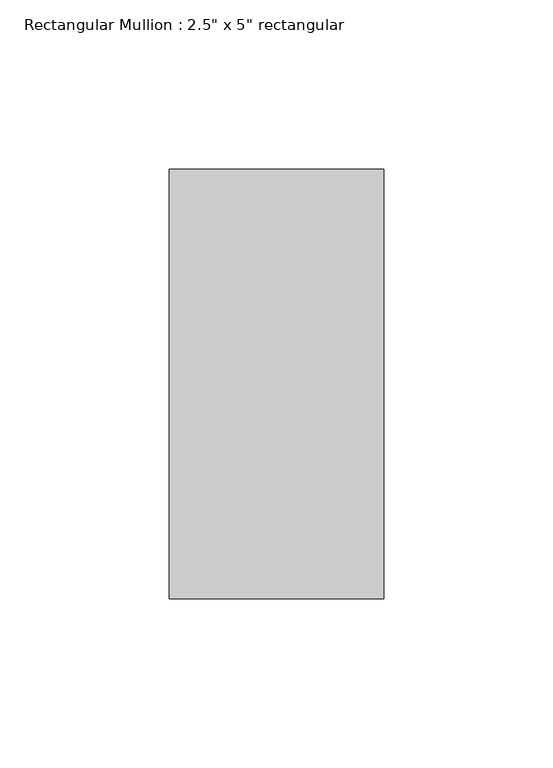
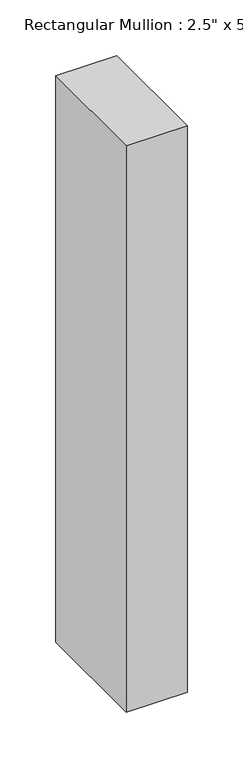
"""IFC4 building model written with IfcOpenShell, lengths in millimetres: member geometry."""

from ifc_helpers import new_model, si_unit, frame, origin, place, context, project, spatial, polyline, outline, extrude, source, transform, mapped, element, save


def member_081e0693(model_context):
    return source(origin(), model_context, "Body", "SweptSolid", [
        extrude(outline(polyline([(0.0, 63.5), (0.0, -63.5), (-63.5, -63.5), (-63.5, 63.5), (0.0, 63.5)])), frame((0.0, 0.0, -622.3), z_axis=(0.0, 0.0, 1.0), x_axis=(1.0, 0.0, 0.0)), (0.0, 0.0, 1.0), 622.3),
    ])


if __name__ == "__main__":
    model = new_model("IFC4")
    model_context = context("Model", 3, world=origin())
    ifc_project = project(units=[si_unit("LENGTHUNIT", "METRE", prefix="MILLI")], contexts=[model_context])
    site = spatial("IfcSite", under=ifc_project)
    building = spatial("IfcBuilding", under=site)
    placement = place(None, origin())
    member_shape = member_081e0693(model_context)
    element("IfcMember", 1, ObjectType="Rectangular Mullion : 2.5\" x 5\" rectangular", at=placement, inside=building, context=model_context, shape_type="MappedRepresentation", body=[
        mapped(member_shape, transform((0.0, 0.0, 0.0), x_axis=(1.0, 0.0, 0.0), y_axis=(0.0, 1.0, 0.0), z_axis=(0.0, 0.0, 1.0))),
    ])
    save(model, "model.ifc")

# Revit data of these elements
# Type "Rectangular Mullion : 2.5\" x 5\" rectangular"
#   built-in parameter 1007304 = 0.416667 (stored number, unit not read)
#   built-in parameter 1007301 = 0.104167 (stored number, unit not read)
#   built-in parameter 1007300 = 0.104167 (stored number, unit not read)
# Element 1 (IfcMember, "Rectangular Mullion : 2.5\" x 5\" rectangular")
#   Materials on its faces: "door black"
# Materials
#   "door black": class "Generic", colour RGB 120 120 120, transparency 0, Cost = 0
